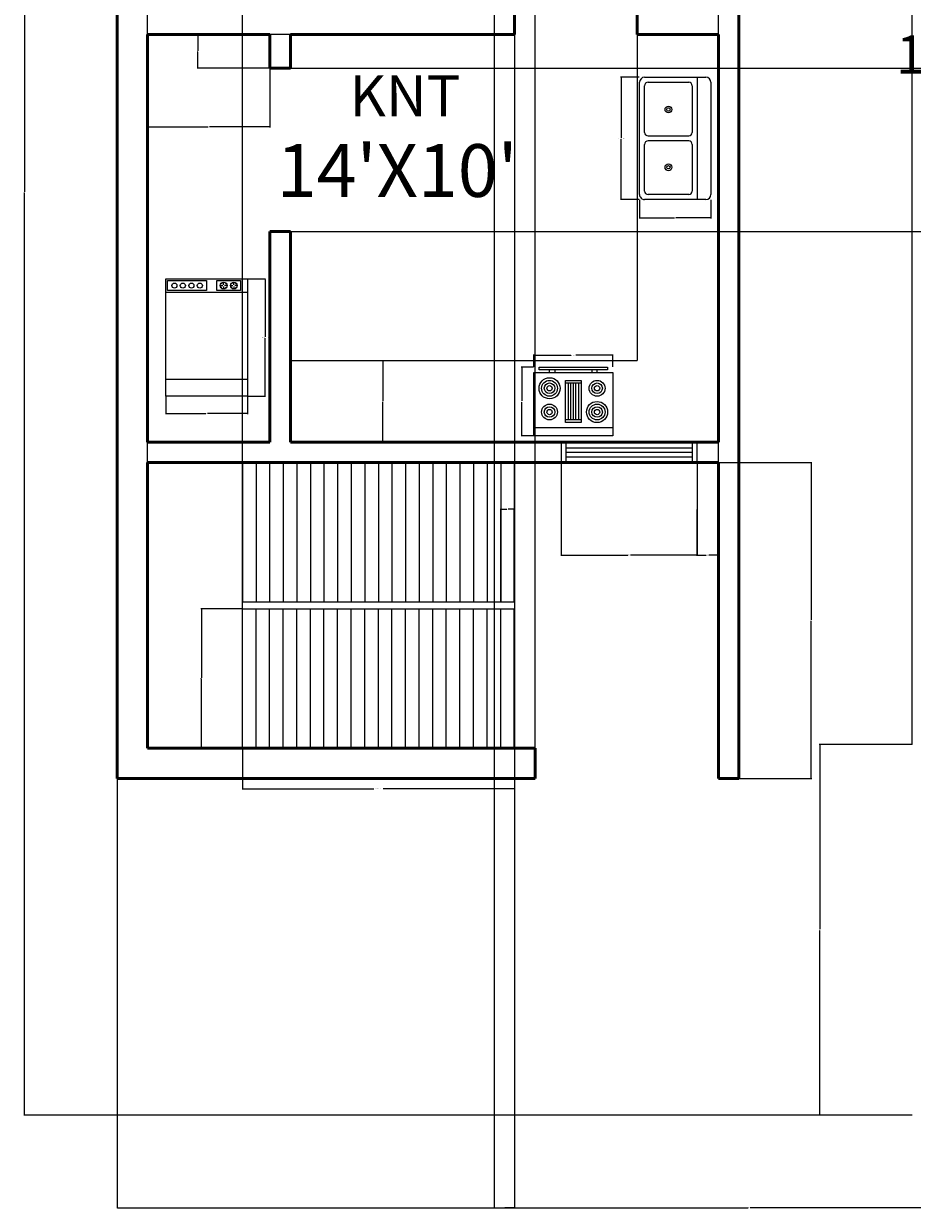
# Model space of a CAD drawing. Units: inches. Extents: x 16 to 443, y 39 to 637.
# Tile 1 of 3: x 16 to 278, y 39 to 387. Entities that reach past the tile are written whole.
import ezdxf

# ---------------------------------------------------------------- set-up
doc = ezdxf.new("R2010")
doc.units = ezdxf.units.IN
for name, color, linetype, lineweight in [('A-ANNO-DIMS', 2, 'Continuous', 18), ('A-AREA-IDEN', 7, 'Continuous', 18), ('A-EQPM', 8, 'Continuous', 18), ('A-FLOR-CASE', 8, 'Continuous', 25), ('A-FLOR-FIXT', 9, 'Continuous', 18), ('A-FLOR-STRS', 7, 'Continuous', 25), ('A-GLAZ', 4, 'Continuous', 18), ('A-WALL', 7, 'Continuous', 50)]:
    doc.layers.add(name, color=color, linetype=linetype, lineweight=lineweight)
doc.styles.get("Standard").update_dxf_attribs({"font": 'arial.ttf'})
doc.dimstyles.get("Standard").update_dxf_attribs({"dimtxt": 0.18, "dimasz": 0.18, "dimexe": 0.18, "dimexo": 0.0625, "dimgap": 0.09, "dimtad": 0, "dimtih": 1, "dimtoh": 1, "dimdec": 4, "dimzin": 0, "dimdsep": 46, "dimtxsty": 'Standard', "dimcen": 0.09, "dimadec": 0, "dimazin": 0, "dimtfac": 1, "dimtdec": 4, "dimtofl": 0, "dimtmove": 0, "dimatfit": 3, "dimfxl": 1, "dimtolj": 1, "dimtzin": 0, "dimarcsym": 0})

# ---------------------------------------------------------------- blocks, each defined once
blk = doc.blocks.new('Sink-double - 36 in top')
for p, q in [((-18, -4), (18, -4)), ((-0.75, -18.5), (-0.75, -6.5)), ((0.75, -6.5), (0.75, -18.5))]:
    blk.add_line(p, q)
for points in [[(-16.5, 0), (16.5, 0)], [(-18, -19.5), (-18, -1.5)], [(18, -1.5), (18, -19.5)], [(-16.5, -18.5), (-16.5, -6.5)], [(-15.5, -5.5), (-1.75, -5.5)], [(1.75, -5.5), (15.5, -5.5)], [(16.5, -6.5), (16.5, -18.5)], [(-1.75, -19.5), (-15.5, -19.5)], [(15.5, -19.5), (1.75, -19.5)], [(16.5, -21), (-16.5, -21)]]:
    blk.add_lwpolyline(points)
for centre, radius in [((-8.5, -12.5), 1), ((-8.5, -12.5), 0.5), ((8.5, -12.5), 1), ((8.5, -12.5), 0.5)]:
    blk.add_circle(centre, radius)
for centre, radius, start, end in [((-16.5, -1.5), 1.5, 90, 180), ((16.5, -1.5), 1.5, 0, 90), ((-15.5, -6.5), 1, 90, 180), ((-1.75, -6.5), 1, 0, 90), ((1.75, -6.5), 1, 90, 180), ((15.5, -6.5), 1, 0, 90), ((-16.5, -19.5), 1.5, 180, 270), ((-15.5, -18.5), 1, 180, 270), ((-1.75, -18.5), 1, 270, 0), ((1.75, -18.5), 1, 180, 270), ((15.5, -18.5), 1, 270, 0), ((16.5, -19.5), 1.5, 270, 0)]:
    blk.add_arc(centre, radius, start, end)
blk = doc.blocks.new('Range-Oven - 30 in top')
for p, q in [((0, -3), (30, -3)), ((12, -6), (18, -6)), ((13, -20), (13, -6)), ((14, -6), (14, -20)), ((15, -20), (15, -6)), ((16, -6), (16, -20)), ((17, -20), (17, -6)), ((18, -20), (12, -20)), ((6, -24), (6, -25)), ((8, -25), (8, -24)), ((22, -25), (22, -24)), ((24, -24), (24, -25))]:
    blk.add_line(p, q)
for points in [[(0, -24), (0, 0), (30, 0), (30, -24)], [(12, -21), (12, -5), (18, -5), (18, -21)], [(2, -26), (2, -25), (28, -25), (28, -26)]]:
    blk.add_lwpolyline(points, close=True)
for centre, radius in [((6, -9), 4), ((6, -9), 3), ((6, -9), 2), ((6, -9), 1), ((24, -9), 3), ((24, -9), 2), ((24, -9), 1), ((6, -18), 3), ((6, -18), 2), ((6, -18), 1), ((24, -18), 4), ((24, -18), 3), ((24, -18), 2), ((24, -18), 1)]:
    blk.add_circle(centre, radius)
blk = doc.blocks.new('Dishwasher')
for p, q in [((16, 32.5), (16.75, 32.5)), ((16.5, 32), (16.2942, 31.7942)), ((16.3156, 33.1843), (16.5, 33)), ((17, 32.75), (17, 33.5)), ((17, 32.25), (17, 31.5)), ((18, 32.5), (17.25, 32.5)), ((17.5, 33), (17.6938, 33.1938)), ((17.7061, 31.7939), (17.5, 32)), ((19, 32.5), (19.75, 32.5)), ((19.5, 32), (19.2942, 31.7942)), ((19.3156, 33.1843), (19.5, 33)), ((20, 32.75), (20, 33.5)), ((20, 32.25), (20, 31.5)), ((21, 32.5), (20.25, 32.5)), ((20.5, 33), (20.6938, 33.1938)), ((20.7061, 31.7939), (20.5, 32)), ((24, 30.5), (0, 30.5)), ((0, 5), (24, 5))]:
    blk.add_line(p, q)
for points in [[(0, 0), (0, 34.5), (24, 34.5), (24, 0)], [(0.5, 31), (0.5, 34), (12, 34), (12, 31)], [(15, 31), (15, 34), (22, 34), (22, 31)]]:
    blk.add_lwpolyline(points, close=True)
for centre, radius in [((2.5, 32.5), 0.75), ((5, 32.5), 0.75), ((7.5, 32.5), 0.75), ((10, 32.5), 0.75), ((17, 32.5), 1), ((20, 32.5), 1)]:
    blk.add_circle(centre, radius)
blk = doc.blocks.new('STAIR-FLIGHT-20-TREADS')
for p, q in [((0, 41), (0, 0)), ((4, 41), (4, 0)), ((8, 41), (8, 0)), ((12, 41), (12, 0)), ((16, 41), (16, 0)), ((20, 41), (20, 0)), ((24, 41), (24, 0)), ((28, 41), (28, 0)), ((32, 41), (32, 0)), ((36, 41), (36, 0)), ((40, 41), (40, 0)), ((44, 41), (44, 0)), ((48, 41), (48, 0)), ((52, 41), (52, 0)), ((56, 41), (56, 0)), ((60, 41), (60, 0)), ((64, 41), (64, 0)), ((68, 41), (68, 0)), ((72, 41), (72, 0)), ((76, 41), (76, 0)), ((80, 41), (80, 0)), ((0, 0), (80.08, 0))]:
    blk.add_line(p, q)
blk = doc.blocks.new('*D31')
at = {"layer": 'A-ANNO-DIMS', "color": 0, "lineweight": -2, "transparency": 16777216}
for p, q in [((80.65, 174.02), (80.65, 161.89)), ((160.73, 174.02), (160.73, 161.89)), ((80.83, 162.07), (119.27, 162.07)), ((160.55, 162.07), (122.1, 162.07))]:
    blk.add_line(p, q, dxfattribs=at)
at = {"layer": 'A-ANNO-DIMS', "color": 0, "transparency": 16777216}
for points in [[(80.83, 162.1), (80.83, 162.04), (80.65, 162.07)], [(160.55, 162.1), (160.55, 162.04), (160.73, 162.07)]]:
    blk.add_solid(points, dxfattribs=at)
at = {"layer": 'Defpoints', "color": 0, "transparency": 16777216}
for p in [(80.65, 174.08), (160.73, 174.08), (160.73, 162.07)]:
    blk.add_point(p, dxfattribs=at)
at = {"layer": 'A-ANNO-DIMS', "color": 0, "transparency": 16777216, "insert": (120.69, 162.07), "char_height": 0.18, "attachment_point": 5}
blk.add_mtext('\\A1;STAIR FLIGHT 80 TYP.', dxfattribs=at)
blk = doc.blocks.new('*D32')
at = {"layer": 'A-ANNO-DIMS', "color": 0, "lineweight": -2, "transparency": 16777216}
for p, q in [((80.58, 215.08), (68.45, 215.08)), ((68.63, 214.9), (68.63, 194.76)), ((68.63, 174.26), (68.63, 194.4)), ((80.58, 174.08), (68.45, 174.08))]:
    blk.add_line(p, q, dxfattribs=at)
at = {"layer": 'A-ANNO-DIMS', "color": 0, "transparency": 16777216}
for points in [[(68.6, 214.9), (68.66, 214.9), (68.63, 215.08)], [(68.6, 174.26), (68.66, 174.26), (68.63, 174.08)]]:
    blk.add_solid(points, dxfattribs=at)
at = {"layer": 'Defpoints', "color": 0, "transparency": 16777216}
for p in [(80.65, 215.08), (68.63, 174.08), (80.65, 174.08)]:
    blk.add_point(p, dxfattribs=at)
at = {"layer": 'A-ANNO-DIMS', "color": 0, "transparency": 16777216, "insert": (68.63, 194.58), "char_height": 0.18, "attachment_point": 5}
blk.add_mtext('\\A1;41 TYP.', dxfattribs=at)
blk = doc.blocks.new('*D35')
at = {"layer": 'A-ANNO-DIMS', "color": 0, "lineweight": -2, "transparency": 16777216}
for p, q in [((197.43, 371.46), (191.92, 371.46)), ((192.1, 371.28), (192.1, 353.65)), ((192.1, 335.64), (192.1, 353.28)), ((197.43, 335.46), (191.92, 335.46))]:
    blk.add_line(p, q, dxfattribs=at)
at = {"layer": 'A-ANNO-DIMS', "color": 0, "transparency": 16777216}
for points in [[(192.07, 371.28), (192.13, 371.28), (192.1, 371.46)], [(192.07, 335.64), (192.13, 335.64), (192.1, 335.46)]]:
    blk.add_solid(points, dxfattribs=at)
at = {"layer": 'Defpoints', "color": 0, "transparency": 16777216}
for p in [(197.5, 371.46), (192.1, 335.46), (197.5, 335.46)]:
    blk.add_point(p, dxfattribs=at)
at = {"layer": 'A-ANNO-DIMS', "color": 0, "transparency": 16777216, "insert": (192.1, 353.46), "char_height": 0.18, "attachment_point": 5}
blk.add_mtext('\\A1;DOUBLE SINK 36', dxfattribs=at)
blk = doc.blocks.new('*D36')
at = {"layer": 'A-ANNO-DIMS', "color": 0, "lineweight": -2, "transparency": 16777216}
for p, q in [((197.5, 335.4), (197.5, 329.88)), ((218.5, 335.4), (218.5, 329.88)), ((197.68, 330.06), (207.79, 330.06)), ((218.32, 330.06), (208.2, 330.06))]:
    blk.add_line(p, q, dxfattribs=at)
at = {"layer": 'A-ANNO-DIMS', "color": 0, "transparency": 16777216}
for points in [[(197.68, 330.09), (197.68, 330.03), (197.5, 330.06)], [(218.32, 330.09), (218.32, 330.03), (218.5, 330.06)]]:
    blk.add_solid(points, dxfattribs=at)
at = {"layer": 'Defpoints', "color": 0, "transparency": 16777216}
for p in [(197.5, 335.46), (218.5, 335.46), (218.5, 330.06)]:
    blk.add_point(p, dxfattribs=at)
at = {"layer": 'A-ANNO-DIMS', "color": 0, "transparency": 16777216, "insert": (208, 330.06), "char_height": 0.18, "attachment_point": 5}
blk.add_mtext('\\A1;21', dxfattribs=at)
blk = doc.blocks.new('*D37')
at = {"layer": 'A-ANNO-DIMS', "color": 0, "lineweight": -2, "transparency": 16777216}
for p, q in [((166.36, 286.22), (166.36, 289.83)), ((166.54, 289.65), (177.32, 289.65)), ((189.48, 289.65), (178.71, 289.65)), ((189.66, 286.22), (189.66, 289.83))]:
    blk.add_line(p, q, dxfattribs=at)
at = {"layer": 'A-ANNO-DIMS', "color": 0, "transparency": 16777216}
for points in [[(166.54, 289.68), (166.54, 289.62), (166.36, 289.65)], [(189.48, 289.68), (189.48, 289.62), (189.66, 289.65)]]:
    blk.add_solid(points, dxfattribs=at)
at = {"layer": 'Defpoints', "color": 0, "transparency": 16777216}
for p in [(166.36, 289.65), (166.36, 286.16), (189.66, 286.16)]:
    blk.add_point(p, dxfattribs=at)
at = {"layer": 'A-ANNO-DIMS', "color": 0, "transparency": 16777216, "insert": (178.01, 289.65), "char_height": 0.18, "attachment_point": 5}
blk.add_mtext('\\A1;RANGE 23', dxfattribs=at)
blk = doc.blocks.new('*D38')
at = {"layer": 'A-ANNO-DIMS', "color": 0, "lineweight": -2, "transparency": 16777216}
for p, q in [((166.3, 286.16), (162.68, 286.16)), ((162.86, 285.98), (162.86, 276.24)), ((162.86, 266.14), (162.86, 275.87)), ((166.3, 265.96), (162.68, 265.96))]:
    blk.add_line(p, q, dxfattribs=at)
at = {"layer": 'A-ANNO-DIMS', "color": 0, "transparency": 16777216}
for points in [[(162.83, 285.98), (162.89, 285.98), (162.86, 286.16)], [(162.83, 266.14), (162.89, 266.14), (162.86, 265.96)]]:
    blk.add_solid(points, dxfattribs=at)
at = {"layer": 'Defpoints', "color": 0, "transparency": 16777216}
for p in [(166.36, 286.16), (162.86, 265.96), (166.36, 265.96)]:
    blk.add_point(p, dxfattribs=at)
at = {"layer": 'A-ANNO-DIMS', "color": 0, "transparency": 16777216, "insert": (162.86, 276.06), "char_height": 0.18, "attachment_point": 5}
blk.add_mtext('\\A1;20', dxfattribs=at)
blk = doc.blocks.new('*D39')
at = {"layer": 'A-ANNO-DIMS', "color": 0, "lineweight": -2, "transparency": 16777216}
for p, q in [((82.19, 312.16), (87.48, 312.16)), ((87.3, 311.98), (87.3, 295.1)), ((87.3, 277.84), (87.3, 294.73)), ((82.19, 277.66), (87.48, 277.66))]:
    blk.add_line(p, q, dxfattribs=at)
at = {"layer": 'A-ANNO-DIMS', "color": 0, "transparency": 16777216}
for points in [[(87.27, 311.98), (87.33, 311.98), (87.3, 312.16)], [(87.27, 277.84), (87.33, 277.84), (87.3, 277.66)]]:
    blk.add_solid(points, dxfattribs=at)
at = {"layer": 'Defpoints', "color": 0, "transparency": 16777216}
for p in [(82.13, 312.16), (87.3, 312.16), (82.13, 277.66)]:
    blk.add_point(p, dxfattribs=at)
at = {"layer": 'A-ANNO-DIMS', "color": 0, "transparency": 16777216, "insert": (87.3, 294.91), "char_height": 0.18, "attachment_point": 5}
blk.add_mtext('\\A1;DISHWASHER 35', dxfattribs=at)
blk = doc.blocks.new('*D40')
at = {"layer": 'A-ANNO-DIMS', "color": 0, "lineweight": -2, "transparency": 16777216}
for p, q in [((58.13, 277.6), (58.13, 272.31)), ((82.13, 277.6), (82.13, 272.31)), ((58.31, 272.49), (69.91, 272.49)), ((81.95, 272.49), (70.35, 272.49))]:
    blk.add_line(p, q, dxfattribs=at)
at = {"layer": 'A-ANNO-DIMS', "color": 0, "transparency": 16777216}
for points in [[(58.31, 272.52), (58.31, 272.46), (58.13, 272.49)], [(81.95, 272.52), (81.95, 272.46), (82.13, 272.49)]]:
    blk.add_solid(points, dxfattribs=at)
at = {"layer": 'Defpoints', "color": 0, "transparency": 16777216}
for p in [(58.13, 277.66), (82.13, 277.66), (82.13, 272.49)]:
    blk.add_point(p, dxfattribs=at)
at = {"layer": 'A-ANNO-DIMS', "color": 0, "transparency": 16777216, "insert": (70.13, 272.49), "char_height": 0.18, "attachment_point": 5}
blk.add_mtext('\\A1;24', dxfattribs=at)
blk = doc.blocks.new('*D45')
at = {"layer": 'A-ANNO-DIMS', "color": 0, "lineweight": -2, "transparency": 16777216}
for p, q in [((43.75, 165.02), (43.75, 38.65)), ((415.75, 66.02), (415.75, 38.65)), ((43.93, 38.83), (229.46, 38.83)), ((415.57, 38.83), (230.04, 38.83))]:
    blk.add_line(p, q, dxfattribs=at)
at = {"layer": 'A-ANNO-DIMS', "color": 0, "transparency": 16777216}
for points in [[(43.93, 38.86), (43.93, 38.8), (43.75, 38.83)], [(415.57, 38.86), (415.57, 38.8), (415.75, 38.83)]]:
    blk.add_solid(points, dxfattribs=at)
at = {"layer": 'Defpoints', "color": 0, "transparency": 16777216}
for p in [(43.75, 165.08), (415.75, 66.08), (415.75, 38.83)]:
    blk.add_point(p, dxfattribs=at)
at = {"layer": 'A-ANNO-DIMS', "color": 0, "transparency": 16777216, "insert": (229.75, 38.83), "char_height": 0.18, "attachment_point": 5}
blk.add_mtext('\\A1;372', dxfattribs=at)
blk = doc.blocks.new('*D46')
at = {"layer": 'A-ANNO-DIMS', "color": 0, "lineweight": -2, "transparency": 16777216}
for p, q in [((43.69, 609.08), (16.32, 609.08)), ((16.5, 608.9), (16.5, 337.76)), ((16.5, 66.26), (16.5, 337.4)), ((277.69, 66.08), (16.32, 66.08))]:
    blk.add_line(p, q, dxfattribs=at)
at = {"layer": 'A-ANNO-DIMS', "color": 0, "transparency": 16777216}
for points in [[(16.47, 608.9), (16.53, 608.9), (16.5, 609.08)], [(16.47, 66.26), (16.53, 66.26), (16.5, 66.08)]]:
    blk.add_solid(points, dxfattribs=at)
at = {"layer": 'Defpoints', "color": 0, "transparency": 16777216}
for p in [(16.5, 609.08), (43.75, 609.08), (277.75, 66.08)]:
    blk.add_point(p, dxfattribs=at)
at = {"layer": 'A-ANNO-DIMS', "color": 0, "transparency": 16777216, "insert": (16.5, 337.58), "char_height": 0.18, "attachment_point": 5}
blk.add_mtext('\\A1;543', dxfattribs=at)
blk = doc.blocks.new('*D47')
at = {"layer": 'A-ANNO-DIMS', "color": 0, "lineweight": -2, "transparency": 16777216}
for p, q in [((174.48, 258.04), (174.48, 230.67)), ((214.41, 258.04), (214.41, 230.67)), ((174.66, 230.85), (194.06, 230.85)), ((214.23, 230.85), (194.84, 230.85))]:
    blk.add_line(p, q, dxfattribs=at)
at = {"layer": 'A-ANNO-DIMS', "color": 0, "transparency": 16777216}
for points in [[(174.66, 230.88), (174.66, 230.82), (174.48, 230.85)], [(214.23, 230.88), (214.23, 230.82), (214.41, 230.85)]]:
    blk.add_solid(points, dxfattribs=at)
at = {"layer": 'Defpoints', "color": 0, "transparency": 16777216}
for p in [(174.48, 258.1), (214.41, 258.1), (174.48, 230.85)]:
    blk.add_point(p, dxfattribs=at)
at = {"layer": 'A-ANNO-DIMS', "color": 0, "transparency": 16777216, "insert": (194.45, 230.85), "char_height": 0.18, "attachment_point": 5}
blk.add_mtext('\\A1;39.93', dxfattribs=at)
blk = doc.blocks.new('*D48')
at = {"layer": 'A-ANNO-DIMS', "color": 0, "lineweight": -2, "transparency": 16777216}
for p, q in [((214.41, 258.04), (214.32, 230.67)), ((220.75, 258.02), (220.65, 230.65)), ((214.5, 230.85), (217.09, 230.84)), ((220.47, 230.83), (217.88, 230.84))]:
    blk.add_line(p, q, dxfattribs=at)
at = {"layer": 'A-ANNO-DIMS', "color": 0, "transparency": 16777216}
for points in [[(214.5, 230.88), (214.5, 230.82), (214.32, 230.85)], [(220.47, 230.86), (220.47, 230.8), (220.65, 230.83)]]:
    blk.add_solid(points, dxfattribs=at)
at = {"layer": 'Defpoints', "color": 0, "transparency": 16777216}
for p in [(214.41, 258.1), (220.75, 258.08), (214.32, 230.85)]:
    blk.add_point(p, dxfattribs=at)
at = {"layer": 'A-ANNO-DIMS', "color": 0, "transparency": 16777216, "insert": (217.49, 230.84), "char_height": 0.18, "attachment_point": 5}
blk.add_mtext('\\A1;6.334', dxfattribs=at)
blk = doc.blocks.new('*D49')
at = {"layer": 'A-ANNO-DIMS', "color": 0, "lineweight": -2, "transparency": 16777216}
for p, q in [((226.75, 165.14), (226.75, 636.51)), ((226.93, 636.33), (252.05, 636.33)), ((277.57, 636.33), (252.45, 636.33)), ((277.75, 175.14), (277.75, 636.51))]:
    blk.add_line(p, q, dxfattribs=at)
at = {"layer": 'A-ANNO-DIMS', "color": 0, "transparency": 16777216}
for points in [[(226.93, 636.36), (226.93, 636.3), (226.75, 636.33)], [(277.57, 636.36), (277.57, 636.3), (277.75, 636.33)]]:
    blk.add_solid(points, dxfattribs=at)
at = {"layer": 'Defpoints', "color": 0, "transparency": 16777216}
for p in [(277.75, 636.33), (277.75, 175.08), (226.75, 165.08)]:
    blk.add_point(p, dxfattribs=at)
at = {"layer": 'A-ANNO-DIMS', "color": 0, "transparency": 16777216, "insert": (252.25, 636.33), "char_height": 0.18, "attachment_point": 5}
blk.add_mtext('\\A1;51', dxfattribs=at)
blk = doc.blocks.new('*D50')
at = {"layer": 'A-ANNO-DIMS', "color": 0, "lineweight": -2, "transparency": 16777216}
for p, q in [((220.81, 258.08), (248.18, 258.08)), ((248, 257.9), (248, 211.76)), ((248, 165.26), (248, 211.4)), ((220.81, 165.08), (248.18, 165.08))]:
    blk.add_line(p, q, dxfattribs=at)
at = {"layer": 'A-ANNO-DIMS', "color": 0, "transparency": 16777216}
for points in [[(247.97, 257.9), (248.03, 257.9), (248, 258.08)], [(247.97, 165.26), (248.03, 165.26), (248, 165.08)]]:
    blk.add_solid(points, dxfattribs=at)
at = {"layer": 'Defpoints', "color": 0, "transparency": 16777216}
for p in [(220.75, 258.08), (220.75, 165.08), (248, 165.08)]:
    blk.add_point(p, dxfattribs=at)
at = {"layer": 'A-ANNO-DIMS', "color": 0, "transparency": 16777216, "insert": (248, 211.58), "char_height": 0.18, "attachment_point": 5}
blk.add_mtext('\\A1;93', dxfattribs=at)
blk = doc.blocks.new('*D51')
at = {"layer": 'A-ANNO-DIMS', "color": 0, "lineweight": -2, "transparency": 16777216}
for p, q in [((277.69, 175.08), (250.32, 175.08)), ((250.5, 174.9), (250.5, 120.76)), ((250.5, 66.26), (250.5, 120.4)), ((277.69, 66.08), (250.32, 66.08))]:
    blk.add_line(p, q, dxfattribs=at)
at = {"layer": 'A-ANNO-DIMS', "color": 0, "transparency": 16777216}
for points in [[(250.47, 174.9), (250.53, 174.9), (250.5, 175.08)], [(250.47, 66.26), (250.53, 66.26), (250.5, 66.08)]]:
    blk.add_solid(points, dxfattribs=at)
at = {"layer": 'Defpoints', "color": 0, "transparency": 16777216}
for p in [(250.5, 175.08), (277.75, 175.08), (277.75, 66.08)]:
    blk.add_point(p, dxfattribs=at)
at = {"layer": 'A-ANNO-DIMS', "color": 0, "transparency": 16777216, "insert": (250.5, 120.58), "char_height": 0.18, "attachment_point": 5}
blk.add_mtext('\\A1;109', dxfattribs=at)
blk = doc.blocks.new('*D58')
at = {"layer": 'A-ANNO-DIMS', "color": 0, "lineweight": -2, "transparency": 16777216}
for p, q in [((160.75, 384.14), (160.75, 636.51)), ((160.93, 636.33), (178.53, 636.33)), ((196.57, 636.33), (178.97, 636.33)), ((196.75, 390.14), (196.75, 636.51))]:
    blk.add_line(p, q, dxfattribs=at)
at = {"layer": 'A-ANNO-DIMS', "color": 0, "transparency": 16777216}
for points in [[(160.93, 636.36), (160.93, 636.3), (160.75, 636.33)], [(196.57, 636.36), (196.57, 636.3), (196.75, 636.33)]]:
    blk.add_solid(points, dxfattribs=at)
at = {"layer": 'Defpoints', "color": 0, "transparency": 16777216}
for p in [(196.75, 636.33), (196.75, 390.08), (160.75, 384.08)]:
    blk.add_point(p, dxfattribs=at)
at = {"layer": 'A-ANNO-DIMS', "color": 0, "transparency": 16777216, "insert": (178.75, 636.33), "char_height": 0.18, "attachment_point": 5}
blk.add_mtext('\\A1;36', dxfattribs=at)
blk = doc.blocks.new('*D59')
at = {"layer": 'A-ANNO-DIMS', "color": 0, "lineweight": -2, "transparency": 16777216}
for p, q in [((154.75, 390.02), (154.75, 38.65)), ((160.75, 384.02), (160.75, 38.65)), ((154.93, 38.83), (157.6, 38.83)), ((160.57, 38.83), (157.9, 38.83))]:
    blk.add_line(p, q, dxfattribs=at)
at = {"layer": 'A-ANNO-DIMS', "color": 0, "transparency": 16777216}
for points in [[(154.93, 38.86), (154.93, 38.8), (154.75, 38.83)], [(160.57, 38.86), (160.57, 38.8), (160.75, 38.83)]]:
    blk.add_solid(points, dxfattribs=at)
at = {"layer": 'Defpoints', "color": 0, "transparency": 16777216}
for p in [(154.75, 390.08), (160.75, 384.08), (154.75, 38.83)]:
    blk.add_point(p, dxfattribs=at)
at = {"layer": 'A-ANNO-DIMS', "color": 0, "transparency": 16777216, "insert": (157.75, 38.83), "char_height": 0.18, "attachment_point": 5}
blk.add_mtext('\\A1;6', dxfattribs=at)
blk = doc.blocks.new('*D60')
at = {"layer": 'A-ANNO-DIMS', "color": 0, "lineweight": -2, "transparency": 16777216}
for p, q in [((166.75, 165.14), (166.75, 636.51)), ((166.93, 636.33), (193.53, 636.33)), ((220.57, 636.33), (193.97, 636.33)), ((220.75, 165.14), (220.75, 636.51))]:
    blk.add_line(p, q, dxfattribs=at)
at = {"layer": 'A-ANNO-DIMS', "color": 0, "transparency": 16777216}
for points in [[(166.93, 636.36), (166.93, 636.3), (166.75, 636.33)], [(220.57, 636.36), (220.57, 636.3), (220.75, 636.33)]]:
    blk.add_solid(points, dxfattribs=at)
at = {"layer": 'Defpoints', "color": 0, "transparency": 16777216}
for p in [(220.75, 636.33), (166.75, 165.08), (220.75, 165.08)]:
    blk.add_point(p, dxfattribs=at)
at = {"layer": 'A-ANNO-DIMS', "color": 0, "transparency": 16777216, "insert": (193.75, 636.33), "char_height": 0.18, "attachment_point": 5}
blk.add_mtext('\\A1;54', dxfattribs=at)
blk = doc.blocks.new('*D61')
at = {"layer": 'A-ANNO-DIMS', "color": 0, "lineweight": -2, "transparency": 16777216}
for p, q in [((52.75, 174.14), (52.75, 636.51)), ((52.93, 636.33), (66.23, 636.33)), ((80.47, 636.33), (67.16, 636.33)), ((80.65, 174.14), (80.65, 636.51))]:
    blk.add_line(p, q, dxfattribs=at)
at = {"layer": 'A-ANNO-DIMS', "color": 0, "transparency": 16777216}
for points in [[(52.93, 636.36), (52.93, 636.3), (52.75, 636.33)], [(80.47, 636.36), (80.47, 636.3), (80.65, 636.33)]]:
    blk.add_solid(points, dxfattribs=at)
at = {"layer": 'Defpoints', "color": 0, "transparency": 16777216}
for p in [(80.65, 636.33), (52.75, 174.08), (80.65, 174.08)]:
    blk.add_point(p, dxfattribs=at)
at = {"layer": 'A-ANNO-DIMS', "color": 0, "transparency": 16777216, "insert": (66.7, 636.33), "char_height": 0.18, "attachment_point": 5}
blk.add_mtext('\\A1;27.897', dxfattribs=at)
blk = doc.blocks.new('*D62')
at = {"layer": 'A-ANNO-DIMS', "color": 0, "lineweight": -2, "transparency": 16777216}
for p, q in [((94.81, 374.08), (443.18, 374.08)), ((443, 373.9), (443, 350.26)), ((443, 326.26), (443, 349.9)), ((94.81, 326.08), (443.18, 326.08))]:
    blk.add_line(p, q, dxfattribs=at)
at = {"layer": 'A-ANNO-DIMS', "color": 0, "transparency": 16777216}
for points in [[(442.97, 373.9), (443.03, 373.9), (443, 374.08)], [(442.97, 326.26), (443.03, 326.26), (443, 326.08)]]:
    blk.add_solid(points, dxfattribs=at)
at = {"layer": 'Defpoints', "color": 0, "transparency": 16777216}
for p in [(94.75, 374.08), (443, 374.08), (94.75, 326.08)]:
    blk.add_point(p, dxfattribs=at)
at = {"layer": 'A-ANNO-DIMS', "color": 0, "transparency": 16777216, "insert": (443, 350.08), "char_height": 0.18, "attachment_point": 5}
blk.add_mtext('\\A1;48', dxfattribs=at)
blk = doc.blocks.new('*D67')
at = {"layer": 'A-ANNO-DIMS', "color": 0, "lineweight": -2, "transparency": 16777216}
for p, q in [((94.81, 288.08), (122.18, 288.08)), ((122, 287.9), (122, 276.26)), ((122, 264.26), (122, 275.9)), ((94.81, 264.08), (122.18, 264.08))]:
    blk.add_line(p, q, dxfattribs=at)
at = {"layer": 'A-ANNO-DIMS', "color": 0, "transparency": 16777216}
for points in [[(121.97, 287.9), (122.03, 287.9), (122, 288.08)], [(121.97, 264.26), (122.03, 264.26), (122, 264.08)]]:
    blk.add_solid(points, dxfattribs=at)
at = {"layer": 'Defpoints', "color": 0, "transparency": 16777216}
for p in [(94.75, 288.08), (94.75, 264.08), (122, 264.08)]:
    blk.add_point(p, dxfattribs=at)
at = {"layer": 'A-ANNO-DIMS', "color": 0, "transparency": 16777216, "insert": (122, 276.08), "char_height": 0.18, "attachment_point": 5}
blk.add_mtext('\\A1;24', dxfattribs=at)
blk = doc.blocks.new('*D68')
at = {"layer": 'A-ANNO-DIMS', "color": 0, "lineweight": -2, "transparency": 16777216}
for p, q in [((94.69, 384.08), (67.32, 384.08)), ((67.5, 383.9), (67.5, 379.26)), ((67.5, 374.26), (67.5, 378.9)), ((94.69, 374.08), (67.32, 374.08))]:
    blk.add_line(p, q, dxfattribs=at)
at = {"layer": 'A-ANNO-DIMS', "color": 0, "transparency": 16777216}
for points in [[(67.47, 383.9), (67.53, 383.9), (67.5, 384.08)], [(67.47, 374.26), (67.53, 374.26), (67.5, 374.08)]]:
    blk.add_solid(points, dxfattribs=at)
at = {"layer": 'Defpoints', "color": 0, "transparency": 16777216}
for p in [(67.5, 384.08), (94.75, 384.08), (94.75, 374.08)]:
    blk.add_point(p, dxfattribs=at)
at = {"layer": 'A-ANNO-DIMS', "color": 0, "transparency": 16777216, "insert": (67.5, 379.08), "char_height": 0.18, "attachment_point": 5}
blk.add_mtext('\\A1;10', dxfattribs=at)
blk = doc.blocks.new('*D69')
at = {"layer": 'A-ANNO-DIMS', "color": 0, "lineweight": -2, "transparency": 16777216}
for p, q in [((52.75, 384.02), (52.75, 356.65)), ((88.75, 384.02), (88.75, 356.65)), ((52.93, 356.83), (70.53, 356.83)), ((88.57, 356.83), (70.97, 356.83))]:
    blk.add_line(p, q, dxfattribs=at)
at = {"layer": 'A-ANNO-DIMS', "color": 0, "transparency": 16777216}
for points in [[(52.93, 356.86), (52.93, 356.8), (52.75, 356.83)], [(88.57, 356.86), (88.57, 356.8), (88.75, 356.83)]]:
    blk.add_solid(points, dxfattribs=at)
at = {"layer": 'Defpoints', "color": 0, "transparency": 16777216}
for p in [(52.75, 384.08), (88.75, 384.08), (52.75, 356.83)]:
    blk.add_point(p, dxfattribs=at)
at = {"layer": 'A-ANNO-DIMS', "color": 0, "transparency": 16777216, "insert": (70.75, 356.83), "char_height": 0.18, "attachment_point": 5}
blk.add_mtext('\\A1;36', dxfattribs=at)
blk = doc.blocks.new('*D70')
at = {"layer": 'A-ANNO-DIMS', "color": 0, "lineweight": -2, "transparency": 16777216}
for p, q in [((156.65, 217.14), (156.65, 244.51)), ((156.83, 244.33), (158.49, 244.33)), ((160.47, 244.33), (158.8, 244.33)), ((160.65, 217.14), (160.65, 244.51))]:
    blk.add_line(p, q, dxfattribs=at)
at = {"layer": 'A-ANNO-DIMS', "color": 0, "transparency": 16777216}
for points in [[(156.83, 244.36), (156.83, 244.3), (156.65, 244.33)], [(160.47, 244.36), (160.47, 244.3), (160.65, 244.33)]]:
    blk.add_solid(points, dxfattribs=at)
at = {"layer": 'Defpoints', "color": 0, "transparency": 16777216}
for p in [(160.65, 244.33), (156.65, 217.08), (160.65, 217.08)]:
    blk.add_point(p, dxfattribs=at)
at = {"layer": 'A-ANNO-DIMS', "color": 0, "transparency": 16777216, "insert": (158.65, 244.33), "char_height": 0.18, "attachment_point": 5}
blk.add_mtext('\\A1;4', dxfattribs=at)

msp = doc.modelspace()

# ---------------------------------------------------------------- linework, layer by layer
at = {"layer": 'A-FLOR-CASE'}
for p, q in [((196.7492, 384.0801), (196.7492, 288.0801)), ((94.7492, 288.0801), (160.7492, 288.0801)), ((160.7492, 288.0801), (196.7492, 288.0801))]:
    msp.add_line(p, q, dxfattribs=at)
at = {"layer": 'A-GLAZ'}
for p, q in [((214.4148, 264.092), (174.4827, 264.092)), ((174.4827, 264.092), (174.4827, 258.1022)), ((175.8137, 264.092), (175.8137, 258.1022)), ((175.8137, 262.4281), (213.0837, 262.4281)), ((213.0837, 258.1022), (213.0837, 264.092)), ((214.4148, 258.1022), (214.4148, 264.092)), ((174.4827, 258.1022), (214.4148, 258.1022)), ((175.8137, 261.0971), (213.0837, 261.0971)), ((175.8137, 259.766), (213.0837, 259.766))]:
    msp.add_line(p, q, dxfattribs=at)
at = {"layer": 'A-WALL'}
for p, q in [((43.7492, 165.0801), (43.7492, 609.0801)), ((160.7492, 384.0801), (160.7492, 450.0801)), ((196.7492, 384.0801), (196.7492, 390.0801)), ((226.7492, 390.0801), (226.7492, 165.0801)), ((52.7492, 384.0801), (88.7492, 384.0801)), ((52.7492, 264.0801), (52.7492, 384.0801)), ((88.7492, 374.0801), (88.7492, 384.0801)), ((94.7492, 374.0801), (94.7492, 384.0801)), ((94.7492, 384.0801), (160.7492, 384.0801)), ((214.7492, 384.0801), (196.7492, 384.0801)), ((214.7492, 384.0801), (220.7492, 384.0801)), ((220.7492, 384.0801), (220.7492, 264.0801)), ((88.7492, 374.0801), (94.7492, 374.0801)), ((88.7492, 264.0801), (88.7492, 326.0801)), ((88.7492, 326.0801), (94.7492, 326.0801)), ((94.7492, 264.0801), (94.7492, 326.0801)), ((52.7492, 264.0801), (88.7492, 264.0801)), ((94.7492, 264.0801), (160.7492, 264.0801)), ((160.7492, 264.0801), (220.7492, 264.0801)), ((52.7492, 174.0801), (52.7492, 258.0801)), ((52.7492, 258.0801), (160.7492, 258.0801)), ((160.7492, 258.0801), (220.7492, 258.0801)), ((220.7492, 258.0801), (220.7492, 165.0801)), ((52.7492, 174.0801), (166.7492, 174.0801)), ((166.7492, 174.0801), (166.7492, 165.0801)), ((43.7492, 165.0801), (166.7492, 165.0801)), ((220.7492, 165.0801), (226.7492, 165.0801))]:
    msp.add_line(p, q, dxfattribs=at)

# ---------------------------------------------------------------- block references
at = {"layer": 'A-EQPM'}
msp.add_blockref('Dishwasher', (58.1259, 277.6626), dxfattribs=at)
at = {"layer": 'A-EQPM', "xscale": 0.776857483580455, "yscale": 0.776857483580455, "zscale": 0.776857483580455, "rotation": 180}
msp.add_blockref('Range-Oven - 30 in top', (189.6644, 265.9569), dxfattribs=at)
at = {"layer": 'A-FLOR-FIXT', "rotation": 270}
msp.add_blockref('Sink-double - 36 in top', (218.4959, 353.4633), dxfattribs=at)
at = {"layer": 'A-FLOR-STRS'}
msp.add_blockref('STAIR-FLIGHT-20-TREADS', (80.646, 217.08), dxfattribs=at)
at = {"layer": 'A-FLOR-STRS', "extrusion": (0, 0, -1), "zscale": -1, "rotation": 180}
msp.add_blockref('STAIR-FLIGHT-20-TREADS', (-80.646, 215.0802), dxfattribs=at)

# ---------------------------------------------------------------- texts
at = {"layer": 'A-AREA-IDEN', "attachment_point": 1}
for s, width, gutter_width, insert, char_height in [('15\'X22\'11.1"', 769.796886, 56.4482, (273.0061, 383.7619), 11.289646), ('KNT', 828.270272, 60.736, (112.1752, 372.0582), 12.1472), ("14'X10'", 1058.116511, 77.5903, (90.7613, 351.7666), 15.51807)]:
    msp.add_mtext_dynamic_manual_height_columns(s, width=width, gutter_width=gutter_width, heights=[0], dxfattribs=dict(at, insert=insert, char_height=char_height))

# ---------------------------------------------------------------- dimensions: what is measured, and where the dimension line sits
at = {"layer": 'A-ANNO-DIMS'}
for base, p1, p2, override, picture, middle in [((80.6458, 636.3301), (52.7492, 174.0801), (80.6458, 174.0801), {"dimdec": 3, "dimlfac": 1, "dimrnd": 0, "dimzin": 0, "dimdsep": 46, "dimlunit": 2}, '*D61', (66.6975, 636.3301)), ((196.7492, 636.3301), (160.7492, 384.0801), (196.7492, 390.0801), {"dimdec": 0, "dimlfac": 1, "dimrnd": 0, "dimzin": 0, "dimdsep": 46, "dimlunit": 2}, '*D58', (178.7492, 636.3301)), ((220.7492, 636.3301), (166.7492, 165.0801), (220.7492, 165.0801), {"dimdec": 0, "dimlfac": 1, "dimrnd": 0, "dimzin": 0, "dimdsep": 46, "dimlunit": 2}, '*D60', (193.7492, 636.3301)), ((277.7492, 636.3301), (226.7492, 165.0801), (277.7492, 175.0801), {"dimdec": 0, "dimlfac": 1, "dimrnd": 0, "dimzin": 0, "dimdsep": 46, "dimlunit": 2}, '*D49', (252.2492, 636.3301)), ((154.7492, 38.8301), (160.7492, 384.0801), (154.7492, 390.0801), {"dimdec": 0, "dimlfac": 1, "dimrnd": 0, "dimzin": 0, "dimdsep": 46, "dimlunit": 2}, '*D59', (157.7492, 38.8301)), ((218.4959, 330.0633), (197.4959, 335.4633), (218.4959, 335.4633), {"dimdec": 0, "dimlfac": 1, "dimrnd": 0, "dimzin": 0, "dimdsep": 46, "dimlunit": 2}, '*D36', (207.9959, 330.0633)), ((82.1259, 272.4876), (58.1259, 277.6626), (82.1259, 277.6626), {"dimdec": 0, "dimlfac": 1, "dimrnd": 0, "dimzin": 0, "dimdsep": 46, "dimlunit": 2}, '*D40', (70.1259, 272.4876)), ((160.6458, 244.3301), (156.6458, 217.0801), (160.6458, 217.0801), {"dimdec": 0, "dimlfac": 1, "dimrnd": 0, "dimzin": 0, "dimdsep": 46, "dimlunit": 2}, '*D70', (158.6458, 244.3301)), ((415.7492, 38.8301), (43.7492, 165.0801), (415.7492, 66.0801), {"dimdec": 0, "dimlfac": 1, "dimrnd": 0, "dimzin": 0, "dimdsep": 46, "dimlunit": 2}, '*D45', (229.7492, 38.8301))]:
    dim = msp.add_linear_dim(base=base, p1=p1, p2=p2, dimstyle='Standard', override=override, dxfattribs=at)
    dim.commit()
    dim.dimension.update_dxf_attribs({"geometry": picture, "text_midpoint": middle})
for base, p1, p2, angle, override, picture, middle in [((16.4992, 609.0801), (277.7492, 66.0801), (43.7492, 609.0801), 90, {"dimdec": 0, "dimlfac": 1, "dimrnd": 0, "dimzin": 0, "dimdsep": 46, "dimlunit": 2}, '*D46', (16.4992, 337.5801)), ((52.7492, 356.8301), (88.7492, 384.0801), (52.7492, 384.0801), 180, {"dimdec": 0, "dimlfac": 1, "dimrnd": 0, "dimzin": 0, "dimdsep": 46, "dimlunit": 2}, '*D69', (70.7492, 356.8301)), ((67.4992, 384.0801), (94.7492, 374.0801), (94.7492, 384.0801), 90, {"dimdec": 0, "dimlfac": 1, "dimrnd": 0, "dimzin": 0, "dimdsep": 46, "dimlunit": 2}, '*D68', (67.4992, 379.0801)), ((442.9992, 374.0801), (94.7492, 326.0801), (94.7492, 374.0801), 90, {"dimdec": 0, "dimlfac": 1, "dimrnd": 0, "dimzin": 0, "dimdsep": 46, "dimlunit": 2}, '*D62', (442.9992, 350.0801)), ((121.9992, 264.0801), (94.7492, 288.0801), (94.7492, 264.0801), 270, {"dimdec": 0, "dimlfac": 1, "dimrnd": 0, "dimzin": 0, "dimdsep": 46, "dimlunit": 2}, '*D67', (121.9992, 276.0801)), ((162.8628, 265.9569), (166.3587, 286.1552), (166.3587, 265.9569), 270, {"dimdec": 0, "dimlfac": 1, "dimrnd": 0, "dimzin": 0, "dimdsep": 46, "dimlunit": 2}, '*D38', (162.8628, 276.056)), ((174.4827, 230.8522), (214.4148, 258.1022), (174.4827, 258.1022), 180, {"dimdec": 2, "dimlfac": 1, "dimrnd": 0, "dimzin": 0, "dimdsep": 46, "dimlunit": 2}, '*D47', (194.4487, 230.8522)), ((214.32, 230.8523), (220.7492, 258.0801), (214.4148, 258.1022), 179.800634, {"dimdec": 3, "dimlfac": 1, "dimrnd": 0, "dimzin": 0, "dimdsep": 46, "dimlunit": 2}, '*D48', (217.4872, 230.8413)), ((247.9992, 165.0801), (220.7492, 258.0801), (220.7492, 165.0801), 270, {"dimdec": 0, "dimlfac": 1, "dimrnd": 0, "dimzin": 0, "dimdsep": 46, "dimlunit": 2}, '*D50', (247.9992, 211.5801)), ((250.4992, 175.0801), (277.7492, 66.0801), (277.7492, 175.0801), 90, {"dimdec": 0, "dimlfac": 1, "dimrnd": 0, "dimzin": 0, "dimdsep": 46, "dimlunit": 2}, '*D51', (250.4992, 120.5801))]:
    dim = msp.add_linear_dim(base=base, p1=p1, p2=p2, angle=angle, dimstyle='Standard', override=override, dxfattribs=at)
    dim.commit()
    dim.dimension.update_dxf_attribs({"geometry": picture, "text_midpoint": middle})
for base, p1, p2, angle, text, picture, middle in [((192.0959, 335.4633), (197.4959, 371.4633), (197.4959, 335.4633), 270, 'DOUBLE SINK <>', '*D35', (192.0959, 353.4633)), ((87.3009060394, 312.1626472422), (82.1259060394, 277.6626472422), (82.1259060394, 312.1626472422), 90, 'DISHWASHER <>', '*D39', (87.3009060394, 294.9126472422)), ((166.3587, 289.651), (189.6644, 286.1552), (166.3587, 286.1552), 180, 'RANGE <>', '*D37', (178.0115, 289.651)), ((68.6332, 174.0801), (80.6458, 215.0801), (80.6458, 174.0801), 270, '<> TYP.', '*D32', (68.6332, 194.5801))]:
    dim = msp.add_linear_dim(base=base, p1=p1, p2=p2, angle=angle, text=text, dimstyle='Standard', override={"dimdec": 0, "dimlfac": 1, "dimrnd": 0, "dimzin": 0, "dimdsep": 46, "dimlunit": 2}, dxfattribs=at)
    dim.commit()
    dim.dimension.update_dxf_attribs({"geometry": picture, "text_midpoint": middle})
dim = msp.add_linear_dim(base=(160.7299, 162.0675), p1=(80.6458, 174.0801), p2=(160.7299, 174.0801), text='STAIR FLIGHT <> TYP.', dimstyle='Standard', override={"dimdec": 0, "dimlfac": 1, "dimrnd": 0, "dimzin": 0, "dimdsep": 46, "dimlunit": 2}, dxfattribs=at)
dim.commit()
dim.dimension.update_dxf_attribs({"geometry": '*D31', "text_midpoint": (120.6878, 162.0675)})

doc.saveas('drawing.dxf')
